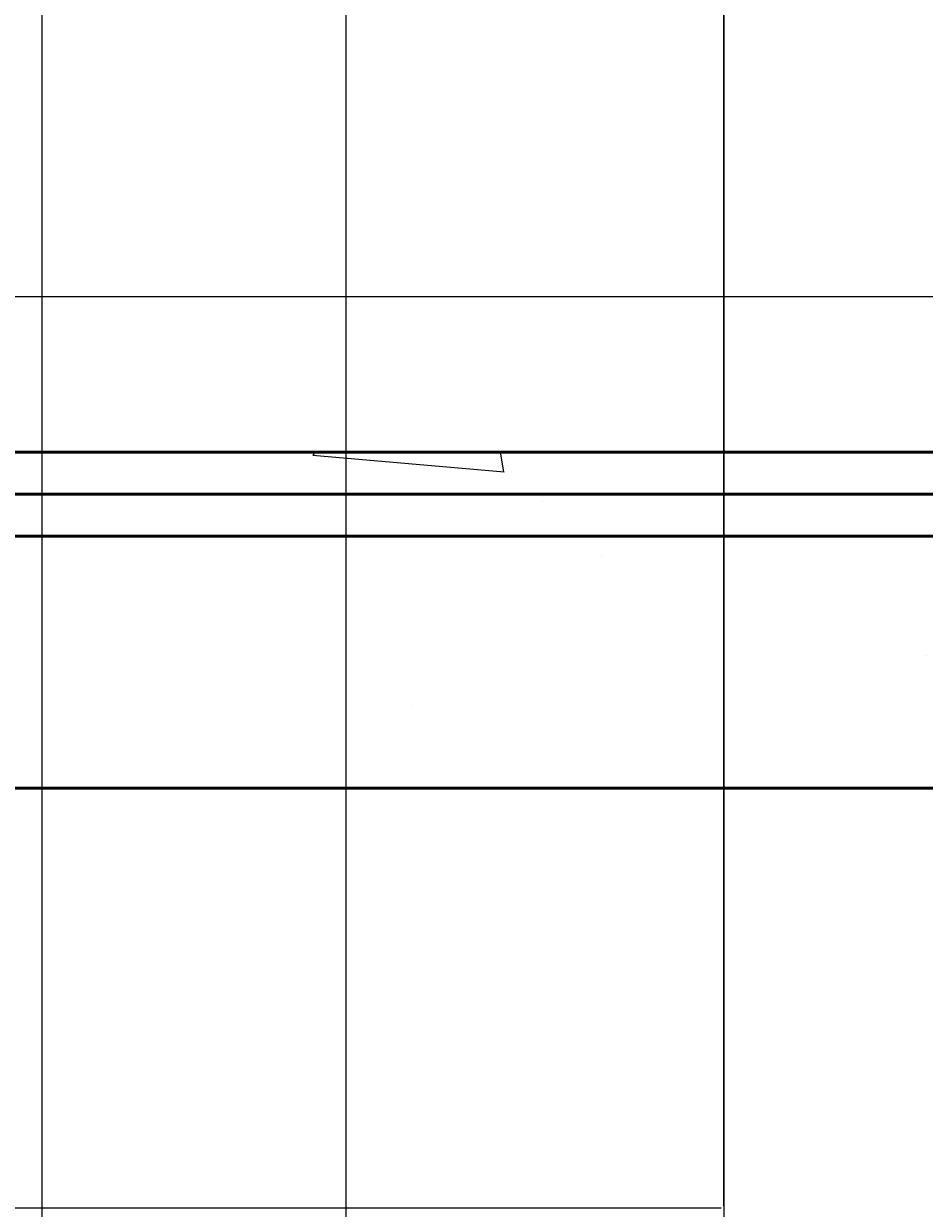
# Model space of a CAD drawing. Units: inches. Extents: x 2812 to 3051, y 1398 to 1659.
# Tile 27 of 65: x 2945 to 2966, y 1472 to 1500. Entities that reach past the tile are written whole.
import ezdxf

# ---------------------------------------------------------------- set-up
doc = ezdxf.new("R2010")
doc.units = ezdxf.units.IN
for name, color, linetype, lineweight in [('A-ANNO-DIMS', 2, 'Continuous', 18), ('S-CONC', 7, 'Continuous', 50), ('S-CONC-PATT', 8, 'Continuous', 18)]:
    doc.layers.add(name, color=color, linetype=linetype, lineweight=lineweight)
doc.styles.get("Standard").update_dxf_attribs({"font": 'arial.ttf'})
doc.dimstyles.get("Standard").update_dxf_attribs({"dimtxt": 0.18, "dimasz": 0.18, "dimexe": 0.18, "dimexo": 0.0625, "dimgap": 0.09, "dimtad": 0, "dimtih": 1, "dimtoh": 1, "dimdec": 4, "dimzin": 0, "dimdsep": 46, "dimtxsty": 'Standard', "dimcen": 0.09, "dimadec": 0, "dimazin": 0, "dimtfac": 1, "dimtdec": 4, "dimtofl": 0, "dimtmove": 0, "dimatfit": 3, "dimfxl": 1, "dimtolj": 1, "dimtzin": 0, "dimarcsym": 0})

# ---------------------------------------------------------------- blocks, each defined once
blk = doc.blocks.new('*D30')
at = {"layer": 'A-ANNO-DIMS', "color": 0, "lineweight": -2, "transparency": 16777216}
for p, q in [((2945.147, 1598.692), (2945.147, 1397.505)), ((2952.385, 1559.757), (2952.385, 1397.505)), ((2945.327, 1397.685), (2948.373, 1397.685)), ((2952.205, 1397.685), (2949.159, 1397.685))]:
    blk.add_line(p, q, dxfattribs=at)
at = {"layer": 'A-ANNO-DIMS', "color": 0, "transparency": 16777216}
for points in [[(2945.327, 1397.715), (2945.327, 1397.655), (2945.147, 1397.685)], [(2952.205, 1397.715), (2952.205, 1397.655), (2952.385, 1397.685)]]:
    blk.add_solid(points, dxfattribs=at)
at = {"layer": 'Defpoints', "color": 0, "transparency": 16777216}
for p in [(2945.147, 1598.754), (2952.385, 1559.82), (2952.385, 1397.685)]:
    blk.add_point(p, dxfattribs=at)
at = {"layer": 'A-ANNO-DIMS', "color": 0, "transparency": 16777216, "insert": (2948.766, 1397.685), "char_height": 0.18, "attachment_point": 5}
blk.add_mtext('\\A1;7.238', dxfattribs=at)
blk = doc.blocks.new('*D31')
at = {"layer": 'A-ANNO-DIMS', "color": 0, "lineweight": -2, "transparency": 16777216}
for p, q in [((2972.272, 1594.192), (2972.272, 1397.505)), ((2961.385, 1559.757), (2961.385, 1397.505)), ((2961.565, 1397.685), (2966.373, 1397.685)), ((2972.092, 1397.685), (2967.283, 1397.685))]:
    blk.add_line(p, q, dxfattribs=at)
at = {"layer": 'A-ANNO-DIMS', "color": 0, "transparency": 16777216}
for points in [[(2961.565, 1397.715), (2961.565, 1397.655), (2961.385, 1397.685)], [(2972.092, 1397.715), (2972.092, 1397.655), (2972.272, 1397.685)]]:
    blk.add_solid(points, dxfattribs=at)
at = {"layer": 'Defpoints', "color": 0, "transparency": 16777216}
for p in [(2972.272, 1594.254), (2961.385, 1559.82), (2972.272, 1397.685)]:
    blk.add_point(p, dxfattribs=at)
at = {"layer": 'A-ANNO-DIMS', "color": 0, "transparency": 16777216, "insert": (2966.828, 1397.685), "char_height": 0.18, "attachment_point": 5}
blk.add_mtext('\\A1;10.887', dxfattribs=at)
blk = doc.blocks.new('*D46')
at = {"layer": 'A-ANNO-DIMS', "color": 0, "lineweight": -2, "transparency": 16777216}
for p, q in [((2941.385, 1487.973), (2941.385, 1397.505)), ((2970.385, 1487.973), (2970.385, 1397.505)), ((2941.565, 1397.685), (2955.664, 1397.685)), ((2970.205, 1397.685), (2956.106, 1397.685))]:
    blk.add_line(p, q, dxfattribs=at)
at = {"layer": 'A-ANNO-DIMS', "color": 0, "transparency": 16777216}
for points in [[(2941.565, 1397.715), (2941.565, 1397.655), (2941.385, 1397.685)], [(2970.205, 1397.715), (2970.205, 1397.655), (2970.385, 1397.685)]]:
    blk.add_solid(points, dxfattribs=at)
at = {"layer": 'Defpoints', "color": 0, "transparency": 16777216}
for p in [(2941.385, 1488.035), (2970.385, 1488.035), (2970.385, 1397.685)]:
    blk.add_point(p, dxfattribs=at)
at = {"layer": 'A-ANNO-DIMS', "color": 0, "transparency": 16777216, "insert": (2955.885, 1397.685), "char_height": 0.18, "attachment_point": 5}
blk.add_mtext('\\A1;29', dxfattribs=at)
blk = doc.blocks.new('*D55')
at = {"layer": 'A-ANNO-DIMS', "color": 0, "lineweight": -2, "transparency": 16777216}
for p, q in [((2850.811, 1493.738), (3051.178, 1493.738)), ((3050.998, 1493.558), (3050.998, 1491.069)), ((3050.998, 1488.215), (3050.998, 1490.705)), ((2850.811, 1488.035), (3051.178, 1488.035))]:
    blk.add_line(p, q, dxfattribs=at)
at = {"layer": 'A-ANNO-DIMS', "color": 0, "transparency": 16777216}
for points in [[(3050.968, 1493.558), (3051.028, 1493.558), (3050.998, 1493.738)], [(3050.968, 1488.215), (3051.028, 1488.215), (3050.998, 1488.035)]]:
    blk.add_solid(points, dxfattribs=at)
at = {"layer": 'Defpoints', "color": 0, "transparency": 16777216}
for p in [(2850.748, 1493.738), (3050.998, 1493.738), (2850.748, 1488.035)]:
    blk.add_point(p, dxfattribs=at)
at = {"layer": 'A-ANNO-DIMS', "color": 0, "transparency": 16777216, "insert": (3050.998, 1490.887), "char_height": 0.18, "attachment_point": 5}
blk.add_mtext('\\A1;5.703', dxfattribs=at)
blk = doc.blocks.new('*D69')
at = {"layer": 'A-ANNO-DIMS', "color": 0, "lineweight": -2, "transparency": 16777216}
for p, q in [((2961.385, 1472.098), (2961.385, 1659.35)), ((2968.956, 1467.81), (2968.956, 1659.35)), ((2961.565, 1659.17), (2964.795, 1659.17)), ((2968.776, 1659.17), (2965.546, 1659.17))]:
    blk.add_line(p, q, dxfattribs=at)
at = {"layer": 'A-ANNO-DIMS', "color": 0, "transparency": 16777216}
for points in [[(2961.565, 1659.2), (2961.565, 1659.14), (2961.385, 1659.17)], [(2968.776, 1659.2), (2968.776, 1659.14), (2968.956, 1659.17)]]:
    blk.add_solid(points, dxfattribs=at)
at = {"layer": 'Defpoints', "color": 0, "transparency": 16777216}
for p in [(2968.956, 1659.17), (2961.385, 1472.035), (2968.956, 1467.747)]:
    blk.add_point(p, dxfattribs=at)
at = {"layer": 'A-ANNO-DIMS', "color": 0, "transparency": 16777216, "insert": (2965.17, 1659.17), "char_height": 0.18, "attachment_point": 5}
blk.add_mtext('\\A1;7.571', dxfattribs=at)
blk = doc.blocks.new('*D77')
at = {"layer": 'A-ANNO-DIMS', "color": 0, "lineweight": -2, "transparency": 16777216}
for p, q in [((2961.322, 1472.035), (2811.806, 1472.035)), ((2811.986, 1471.855), (2811.986, 1461.436)), ((2811.986, 1450.654), (2811.986, 1461.073)), ((2963.812, 1450.474), (2811.806, 1450.474))]:
    blk.add_line(p, q, dxfattribs=at)
at = {"layer": 'A-ANNO-DIMS', "color": 0, "transparency": 16777216}
for points in [[(2811.956, 1471.855), (2812.016, 1471.855), (2811.986, 1472.035)], [(2811.956, 1450.654), (2812.016, 1450.654), (2811.986, 1450.474)]]:
    blk.add_solid(points, dxfattribs=at)
at = {"layer": 'Defpoints', "color": 0, "transparency": 16777216}
for p in [(2811.986, 1472.035), (2961.385, 1472.035), (2963.874, 1450.474)]:
    blk.add_point(p, dxfattribs=at)
at = {"layer": 'A-ANNO-DIMS', "color": 0, "transparency": 16777216, "insert": (2811.986, 1461.255), "char_height": 0.18, "attachment_point": 5}
blk.add_mtext('\\A1;21.56', dxfattribs=at)

msp = doc.modelspace()

# ---------------------------------------------------------------- hatches: boundary and pattern name
at = {"layer": 'S-CONC-PATT'}
h = msp.add_hatch(dxfattribs=at)
h.set_pattern_fill('AR-SAND', color=256, scale=0.3)
h.paths.add_polyline_path([(3036.3849, 1416.0354), (3027.3849, 1416.0354), (2826.3849, 1416.0354), (2826.3849, 1410.0354), (2835.3849, 1410.0354), (3036.3849, 1410.0354)])
h.paths.add_polyline_path([(2970.3849, 1488.0354), (2969.3849, 1488.0354), (2941.3849, 1488.0354), (2941.3849, 1482.0354), (2970.3849, 1482.0354)])
h.paths.add_polyline_path([(3036.3849, 1488.0354), (3035.3849, 1488.0354), (3006.3849, 1488.0354), (3006.3849, 1482.0354), (3027.3849, 1482.0354), (3036.3849, 1482.0354)])
h.paths.add_polyline_path([(3034.3849, 1490.0354), (3008.3849, 1490.0354), (3008.3849, 1489.0354), (3034.3849, 1489.0354)])
h.paths.add_polyline_path([(3035.3849, 1489.0354), (3034.3849, 1489.0354), (3007.3849, 1489.0354), (3007.3849, 1488.0354), (3035.3849, 1488.0354)])
h.paths.add_polyline_path([(2968.3849, 1490.0354), (2943.3849, 1490.0354), (2943.3849, 1489.0354), (2968.3849, 1489.0354)])
h.paths.add_polyline_path([(2969.3849, 1489.0354), (2968.3849, 1489.0354), (2942.3849, 1489.0354), (2942.3849, 1488.0354), (2969.3849, 1488.0354)])
h.paths.add_polyline_path([(2896.3849, 1488.0354), (2826.3849, 1488.0354), (2826.3849, 1482.0354), (2896.3849, 1482.0354)])
h.paths.add_polyline_path([(2895.3849, 1489.0354), (2894.3849, 1489.0354), (2827.3849, 1489.0354), (2827.3849, 1488.0354), (2895.3849, 1488.0354)])
h.paths.add_polyline_path([(2894.3849, 1490.0354), (2828.3849, 1490.0354), (2828.3849, 1489.0354), (2894.3849, 1489.0354)])
h = msp.add_hatch(dxfattribs=at)
h.set_pattern_fill('AR-CONC', color=256, scale=0.3)
h.paths.add_polyline_path([(2896.3849, 1488.0354), (2826.3849, 1488.0354), (2826.3849, 1482.0354), (2896.3849, 1482.0354)])
h.paths.add_polyline_path([(2970.3849, 1488.0354), (2941.3849, 1488.0354), (2941.3849, 1482.0354), (2970.3849, 1482.0354)])
h.paths.add_polyline_path([(2968.3849, 1490.0354), (2943.3849, 1490.0354), (2943.3849, 1489.0354), (2968.3849, 1489.0354)])
h.paths.add_polyline_path([(2969.3849, 1489.0354), (2968.3849, 1489.0354), (2943.3849, 1489.0354), (2942.3849, 1489.0354), (2942.3849, 1488.0354), (2969.3849, 1488.0354)])
h.paths.add_polyline_path([(3036.3849, 1488.0354), (3035.3849, 1488.0354), (3006.3849, 1488.0354), (3006.3849, 1482.0354), (3027.3849, 1482.0354), (3036.3849, 1482.0354)])
h.paths.add_polyline_path([(3035.3849, 1489.0354), (3034.3849, 1489.0354), (3007.3849, 1489.0354), (3007.3849, 1488.0354), (3035.3849, 1488.0354)])
h.paths.add_polyline_path([(3034.3849, 1490.0354), (3008.3849, 1490.0354), (3008.3849, 1489.0354), (3034.3849, 1489.0354)])
h.paths.add_polyline_path([(2895.3849, 1489.0354), (2894.3849, 1489.0354), (2827.3849, 1489.0354), (2827.3849, 1488.0354), (2895.3849, 1488.0354)])
h.paths.add_polyline_path([(2894.3849, 1490.0354), (2828.3849, 1490.0354), (2828.3849, 1489.0354), (2894.3849, 1489.0354)])

# ---------------------------------------------------------------- linework, layer by layer
at = {"layer": 'S-CONC'}
for p, q in [((3034.3849, 1490.0354), (2850.7485, 1490.0354)), ((2850.7485, 1489.0354), (3035.3849, 1489.0354)), ((2850.7485, 1488.0354), (3036.3849, 1488.0354)), ((2850.7485, 1482.0354), (3027.3849, 1482.0354))]:
    msp.add_line(p, q, dxfattribs=at)

# ---------------------------------------------------------------- dimensions: what is measured, and where the dimension line sits
at = {"layer": 'A-ANNO-DIMS'}
for base, p1, p2, override, picture, middle in [((2968.9558, 1659.17), (2961.3849, 1472.0354), (2968.9558, 1467.7474), {"dimdec": 3, "dimlfac": 1, "dimrnd": 0, "dimzin": 0, "dimdsep": 46, "dimlunit": 2}, '*D69', (2965.1704, 1659.17)), ((2952.3849, 1397.6854), (2945.1467, 1598.7541), (2952.3849, 1559.82), {"dimdec": 3, "dimlfac": 1, "dimrnd": 0, "dimzin": 0, "dimdsep": 46, "dimlunit": 2}, '*D30', (2948.7658, 1397.6854)), ((2972.2716, 1397.6854), (2961.3849, 1559.82), (2972.2716, 1594.2541), {"dimdec": 3, "dimlfac": 1, "dimrnd": 0, "dimzin": 0, "dimdsep": 46, "dimlunit": 2}, '*D31', (2966.8282, 1397.6854)), ((2970.3849, 1397.6854), (2941.3849, 1488.0354), (2970.3849, 1488.0354), {"dimdec": 0, "dimlfac": 1, "dimrnd": 0, "dimzin": 0, "dimdsep": 46, "dimlunit": 2}, '*D46', (2955.8849, 1397.6854))]:
    dim = msp.add_linear_dim(base=base, p1=p1, p2=p2, dimstyle='Standard', override=override, dxfattribs=at)
    dim.commit()
    dim.dimension.update_dxf_attribs({"geometry": picture, "text_midpoint": middle})
for base, p1, p2, override, picture, middle in [((3050.998, 1493.7383), (2850.7485, 1488.0354), (2850.7485, 1493.7383), {"dimdec": 3, "dimlfac": 1, "dimrnd": 0, "dimzin": 0, "dimdsep": 46, "dimlunit": 2}, '*D55', (3050.998, 1490.8868)), ((2811.9855, 1472.0354), (2963.8741, 1450.4738), (2961.3849, 1472.0354), {"dimdec": 2, "dimlfac": 1, "dimrnd": 0, "dimzin": 0, "dimdsep": 46, "dimlunit": 2}, '*D77', (2811.9855, 1461.2546))]:
    dim = msp.add_linear_dim(base=base, p1=p1, p2=p2, angle=90, dimstyle='Standard', override=override, dxfattribs=at)
    dim.commit()
    dim.dimension.update_dxf_attribs({"geometry": picture, "text_midpoint": middle})

doc.saveas('drawing.dxf')
